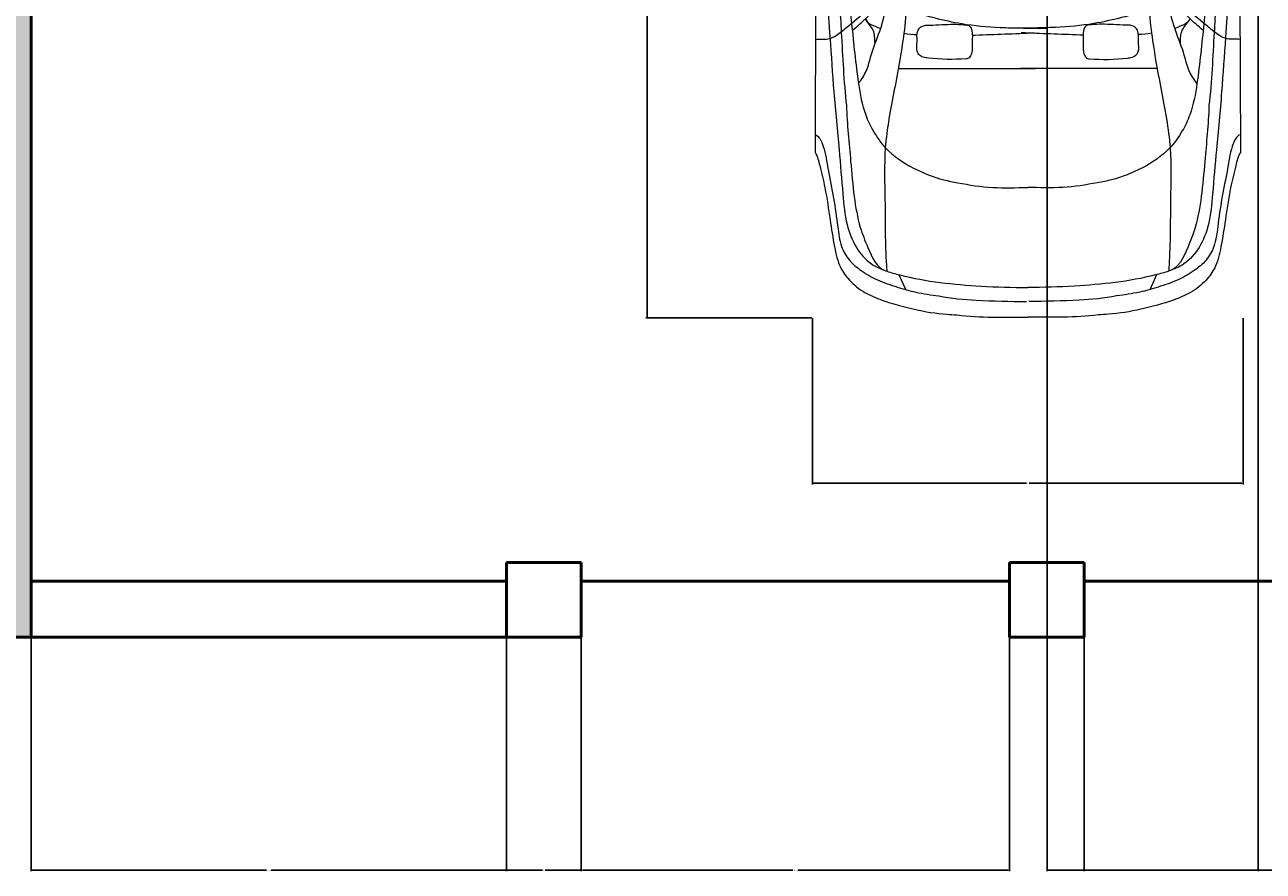
# Model space of a CAD drawing. Units: inches. Extents: x 383 to 970, y 275 to 1088.
# Tile 2 of 11: x 650 to 849, y 275 to 410. Entities that reach past the tile are written whole.
import ezdxf

# ---------------------------------------------------------------- set-up
doc = ezdxf.new("R2010")
doc.units = ezdxf.units.IN
doc.header["$MEASUREMENT"] = 0
for name, color, linetype, lineweight in [('A-ANNO-DIMS', 2, 'Continuous', 18), ('A-COLS', 7, 'Continuous', 50), ('A-EQPM-VEHI', 8, 'Continuous', 13), ('A-WALL', 7, 'Continuous', 50)]:
    doc.layers.add(name, color=color, linetype=linetype, lineweight=lineweight)
doc.layers.add('A-WALL-PATT', color=251, linetype='Continuous', lineweight=13, true_color=0x636466)
doc.styles.get("Standard").update_dxf_attribs({"font": 'arial.ttf'})
doc.dimstyles.get("Standard").update_dxf_attribs({"dimtxt": 0.18, "dimasz": 0.18, "dimexe": 0.18, "dimexo": 0.0625, "dimgap": 0.09, "dimtad": 0, "dimtih": 1, "dimtoh": 1, "dimdec": 4, "dimzin": 0, "dimdsep": 46, "dimtxsty": 'Standard', "dimcen": 0.09, "dimadec": 0, "dimazin": 0, "dimtfac": 1, "dimtdec": 4, "dimtofl": 0, "dimtmove": 0, "dimatfit": 3, "dimfxl": 1, "dimtolj": 1, "dimtzin": 0, "dimarcsym": 0})

# ---------------------------------------------------------------- blocks, each defined once
blk = doc.blocks.new('A$C242571DA')
for p, q in [((1714.3, 1732.5), (3817.1, 1739.9)), ((3474.6, 1401.1), (3474.6, 843)), ((4315.2, 1398), (4377.3, 1370.5)), ((3474.6, 345.6), (3474.6, 903.8)), ((4315.2, 348.7), (4377.3, 376.3)), ((1714.3, 14.2), (3817.1, 6.9))]:
    blk.add_line(p, q)
for points, knots in [([(3356.5, 1739.4), (3354.9, 1719.2), (3360.8, 1678.2), (3324, 1631.5), (3255.4, 1544.3), (3187.1, 1476.2), (3125.2, 1432.2)], [0, 0, 0, 0, 0.0597371, 0.1139981, 0.1672498, 0.3938869, 0.3938869, 0.3938869, 0.3938869]), ([(3745.3, 1736.8), (3748.5, 1730.1), (3764.2, 1717.1), (3811.5, 1698.6), (3894.7, 1686.7), (4002.9, 1663.2), (4107.9, 1648.7), (4195.8, 1638.3), (4258.6, 1603.2), (4302.1, 1549.7), (4339.9, 1483.8), (4365.2, 1407.6), (4389.6, 1324.4), (4397.9, 1266.9), (4401.8, 1235.2)], [0, 0, 0, 0, 0.0219205, 0.0572122, 0.1522539, 0.2718866, 0.3894011, 0.4710097, 0.5346344, 0.5986698, 0.6733118, 0.758696, 0.8351341, 0.9293726, 0.9293726, 0.9293726, 0.9293726]), ([(3817.1, 1739.9), (3833.2, 1729.7), (3882.9, 1718.2), (3973.3, 1695.2), (4085.1, 1680.5), (4193.8, 1662.8), (4280.6, 1644.3), (4343.9, 1598.1), (4390, 1540.3), (4427.4, 1448.7), (4457.8, 1336.6), (4475.7, 1233.4), (4478.4, 1175.1), (4479.3, 1161.6)], [0, 0, 0, 0, 0.056668, 0.14946, 0.28161, 0.392935, 0.481686, 0.542967, 0.622845, 0.69797, 0.833643, 0.965665, 1.00577, 1.00577, 1.00577, 1.00577]), ([(2984.7, 1695.8), (3051, 1695.6), (3172.1, 1691.3), (3367.4, 1677.6), (3575.2, 1664.3), (3788.2, 1643.6), (3968, 1628.1), (4103.8, 1616.8), (4203.6, 1578.1), (4271.8, 1519.5), (4300.6, 1452.1), (4341.7, 1305.3), (4361.8, 1111.2), (4367.5, 936.8), (4367.5, 873.4)], [0, 0, 0, 0, 0.198873, 0.363323, 0.587433, 0.823543, 1.004622, 1.129816, 1.230113, 1.320655, 1.388577, 1.443334, 1.771447, 1.958652, 1.958652, 1.958652, 1.958652]), ([(2695.2, 1655.3), (2829.9, 1655.3), (3041.2, 1651.4), (3351.3, 1630.7), (3527.5, 1623.2), (3626.6, 1612)], [0, 0, 0, 0, 0.4042759, 0.6333827, 0.9326252, 0.9326252, 0.9326252, 0.9326252]), ([(3535.9, 1563.1), (3520.1, 1550.9), (3484.4, 1526.1), (3408.2, 1510.9), (3323.4, 1473.1), (3207.9, 1445), (3072.6, 1422.2), (2866.9, 1404.6), (2626.4, 1412.9), (2396.7, 1410.8), (2200.9, 1416.9), (2001.3, 1438.2), (1732.1, 1525.9), (1527.9, 1578.9), (1407.5, 1610.7)], [0, 0, 0, 0, 0.05975, 0.126928, 0.230034, 0.336675, 0.482225, 0.641324, 0.954906, 1.203173, 1.330375, 1.542773, 1.802261, 2.175545, 2.175545, 2.175545, 2.175545]), ([(2861.6, 1607.5), (2921.1, 1607.3), (3047.2, 1600.8), (3191.4, 1602), (3356.6, 1584.1), (3498.3, 1570.6), (3623.2, 1549.4), (3664.1, 1533.3)], [0, 0, 0, 0, 0.1783018, 0.3787173, 0.431954, 0.6762374, 0.8077184, 0.8077184, 0.8077184, 0.8077184]), ([(3319, 1587.1), (3303.3, 1568.1), (3256.9, 1516.7), (3206.7, 1467.3), (3171.4, 1439.5)], [0, 0, 0, 0, 1.868162, 5.271297, 5.271297, 5.271297, 5.271297]), ([(3626.6, 1612), (3702.5, 1609.1), (3826.2, 1596.8), (3991.4, 1583.2), (4111.7, 1562.4), (4212.2, 1522.7), (4290.4, 1488), (4300.7, 1447.5)], [0, 0, 0, 0, 0.2277977, 0.3719478, 0.4996814, 0.5863441, 0.709615, 0.709615, 0.709615, 0.709615]), ([(3275.5, 1532.8), (3287.5, 1528.3), (3299.8, 1504.9), (3308.4, 1482.5), (3311.7, 1472.6)], [0, 0, 0, 0, 0.983949, 1.771691, 1.771691, 1.771691, 1.771691]), ([(3372.2, 1495.3), (3354.4, 1496.8), (3316, 1494.7), (3291.6, 1525.8), (3275.5, 1532.8)], [0, 0, 0, 0, 0.0535488, 0.1060573, 0.1060573, 0.1060573, 0.1060573]), ([(3664.1, 1533.3), (3687, 1526), (3734.8, 1502.3), (3816.7, 1444.8), (3884.1, 1342.9), (3925.1, 1239.9), (3937.3, 1177), (3940.4, 1157.6)], [0, 0, 0, 0, 0.0720749, 0.1581284, 0.2958089, 0.4262456, 0.4842292, 0.4842292, 0.4842292, 0.4842292]), ([(1909.8, 1424.9), (1933.5, 1418.7), (1995.6, 1407.6), (2094.4, 1385.8), (2211.8, 1377.1), (2419, 1366.9), (2704.7, 1366.5), (3032.7, 1354.2), (3316.2, 1371), (3558.7, 1415.9), (3789.1, 1461.7), (4028.9, 1452.9), (4196.2, 1455.2), (4292.7, 1447.9), (4300.7, 1447.5)], [0, 0, 0, 0, 0.073325, 0.188896, 0.303039, 0.425821, 0.811242, 1.159737, 1.41058, 1.660623, 1.899627, 2.11145, 2.377727, 2.401703, 2.401703, 2.401703, 2.401703]), ([(3231.5, 1368.3), (3240.8, 1356.2), (3253.1, 1315.7), (3271.9, 1240.7), (3297.9, 1127.9), (3310.5, 974.6), (3311.2, 858.3), (3311.6, 794.4)], [0, 0, 0, 0, 0.0451009, 0.1211996, 0.2308505, 0.385263, 0.5739042, 0.5739042, 0.5739042, 0.5739042]), ([(3294.8, 1174.5), (3294.8, 1207.4), (3299.6, 1249.5), (3298.3, 1303.9), (3326.3, 1329), (3363.9, 1320.7), (3399.3, 1329.3), (3422.1, 1315.7), (3430.7, 1297.9), (3438.7, 1234.2), (3439.6, 1174.4), (3434.7, 1112.2), (3418.9, 1102), (3395.9, 1098.6), (3362.6, 1100.9), (3331.1, 1096.6), (3298.8, 1107.6), (3297.3, 1140.3), (3294.8, 1160.9), (3294.8, 1174.5)], [0, 0, 0, 0, 0.0969044, 0.1295913, 0.1506192, 0.1985921, 0.2360698, 0.2557908, 0.2719711, 0.2929882, 0.44406, 0.4519132, 0.4720918, 0.4918599, 0.5228758, 0.5707096, 0.5892096, 0.6145759, 0.654681, 0.654681, 0.654681, 0.654681]), ([(4401.8, 1235.2), (4411.9, 1185.3), (4421.6, 1065.8), (4424.1, 946.5), (4424.1, 878)], [0, 0, 0, 0, 0.1502861, 0.3522699, 0.3522699, 0.3522699, 0.3522699]), ([(3940.4, 1157.6), (3949.9, 1111), (3964.3, 1016.4), (3960.5, 921), (3959.8, 873.4)], [0, 0, 0, 0, 0.140379, 0.2808468, 0.2808468, 0.2808468, 0.2808468]), ([(3339.2, 1099), (3339.1, 1094.8), (3336.4, 1010.6), (3333.2, 926.3), (3330, 846.2)], [11.235438, 11.235438, 11.235438, 11.235438, 11.552536, 17.586883, 17.586883, 17.586883, 17.586883]), ([(3231.5, 378.5), (3240.8, 390.5), (3253.1, 431), (3271.9, 506.1), (3297.9, 618.9), (3310.5, 772.1), (3311.2, 888.4), (3311.6, 952.4)], [0, 0, 0, 0, 0.0451009, 0.1211996, 0.2308505, 0.385263, 0.5739042, 0.5739042, 0.5739042, 0.5739042]), ([(2984.7, 51), (3051, 51.1), (3172.1, 55.5), (3367.4, 69.2), (3575.2, 82.5), (3788.2, 103.1), (3968, 118.7), (4103.8, 130), (4203.6, 168.6), (4271.8, 227.3), (4300.6, 294.7), (4341.7, 441.5), (4361.8, 635.5), (4367.5, 809.9), (4367.5, 873.4)], [0, 0, 0, 0, 0.198873, 0.363323, 0.587433, 0.823543, 1.004622, 1.129816, 1.230113, 1.320655, 1.388577, 1.443334, 1.771447, 1.958652, 1.958652, 1.958652, 1.958652]), ([(3339.2, 647.8), (3339.1, 652), (3336.4, 736.2), (3333.2, 820.5), (3330, 900.6)], [11.235438, 11.235438, 11.235438, 11.235438, 11.552536, 17.586883, 17.586883, 17.586883, 17.586883]), ([(3940.4, 589.1), (3949.9, 635.7), (3964.3, 730.4), (3960.5, 825.8), (3959.8, 873.4)], [0, 0, 0, 0, 0.140379, 0.2808468, 0.2808468, 0.2808468, 0.2808468]), ([(4401.8, 511.5), (4411.9, 561.5), (4421.6, 681), (4424.1, 800.3), (4424.1, 868.8)], [0, 0, 0, 0, 0.1502861, 0.3522699, 0.3522699, 0.3522699, 0.3522699]), ([(3294.8, 572.3), (3294.8, 539.4), (3299.6, 497.2), (3298.3, 442.9), (3326.3, 417.8), (3363.9, 426), (3399.3, 417.5), (3422.1, 431), (3430.7, 448.9), (3438.7, 512.5), (3439.6, 572.4), (3434.7, 634.6), (3418.9, 644.7), (3395.9, 648.2), (3362.6, 645.9), (3331.1, 650.1), (3298.8, 639.2), (3297.3, 606.5), (3294.8, 585.9), (3294.8, 572.3)], [0, 0, 0, 0, 0.0969044, 0.1295913, 0.1506192, 0.1985921, 0.2360698, 0.2557908, 0.2719711, 0.2929882, 0.44406, 0.4519132, 0.4720918, 0.4918599, 0.5228758, 0.5707096, 0.5892096, 0.6145759, 0.654681, 0.654681, 0.654681, 0.654681]), ([(3664.1, 213.5), (3687, 220.8), (3734.8, 244.4), (3816.7, 302), (3884.1, 403.8), (3925.1, 506.9), (3937.3, 569.7), (3940.4, 589.1)], [0, 0, 0, 0, 0.0720749, 0.1581284, 0.2958089, 0.4262456, 0.4842292, 0.4842292, 0.4842292, 0.4842292]), ([(3817.1, 6.9), (3833.2, 17), (3882.9, 28.6), (3973.3, 51.5), (4085.1, 66.3), (4193.8, 84), (4280.6, 102.4), (4343.9, 148.6), (4390, 206.4), (4427.4, 298), (4457.8, 410.1), (4475.7, 513.3), (4478.4, 571.6), (4479.3, 585.2)], [0, 0, 0, 0, 0.056668, 0.14946, 0.28161, 0.392935, 0.481686, 0.542967, 0.622845, 0.69797, 0.833643, 0.965665, 1.00577, 1.00577, 1.00577, 1.00577]), ([(3745.3, 10), (3748.5, 16.7), (3764.2, 29.7), (3811.5, 48.1), (3894.7, 60.1), (4002.9, 83.6), (4107.9, 98), (4195.8, 108.4), (4258.6, 143.5), (4302.1, 197), (4339.9, 262.9), (4365.2, 339.2), (4389.6, 422.4), (4397.9, 479.8), (4401.8, 511.5)], [0, 0, 0, 0, 0.0219205, 0.0572122, 0.1522539, 0.2718866, 0.3894011, 0.4710097, 0.5346344, 0.5986698, 0.6733118, 0.758696, 0.8351341, 0.9293726, 0.9293726, 0.9293726, 0.9293726]), ([(1909.8, 321.9), (1933.5, 328.1), (1995.6, 339.2), (2094.4, 361), (2211.8, 369.6), (2419, 379.8), (2704.7, 380.3), (3032.7, 392.6), (3316.2, 375.8), (3558.7, 330.9), (3789.1, 285.1), (4028.9, 293.9), (4196.2, 291.5), (4292.7, 298.8), (4300.7, 299.2)], [0, 0, 0, 0, 0.073325, 0.188896, 0.303039, 0.425821, 0.811242, 1.159737, 1.41058, 1.660623, 1.899627, 2.11145, 2.377727, 2.401703, 2.401703, 2.401703, 2.401703]), ([(3535.9, 183.7), (3520.1, 195.9), (3484.4, 220.6), (3408.2, 235.8), (3323.4, 273.7), (3207.9, 301.8), (3072.6, 324.6), (2866.9, 342.1), (2626.4, 333.8), (2396.7, 335.9), (2200.9, 329.9), (2001.3, 308.6), (1732.1, 220.8), (1527.9, 167.8), (1407.5, 136)], [0, 0, 0, 0, 0.05975, 0.126928, 0.230034, 0.336675, 0.482225, 0.641324, 0.954906, 1.203173, 1.330375, 1.542773, 1.802261, 2.175545, 2.175545, 2.175545, 2.175545]), ([(3356.5, 7.4), (3354.9, 27.5), (3360.8, 68.5), (3324, 115.2), (3255.4, 202.5), (3187.1, 270.5), (3125.2, 314.6)], [0, 0, 0, 0, 0.0597371, 0.1139981, 0.1672498, 0.3938869, 0.3938869, 0.3938869, 0.3938869]), ([(3319, 159.7), (3303.3, 178.6), (3256.9, 230), (3206.7, 279.5), (3171.4, 307.2)], [0, 0, 0, 0, 1.868162, 5.271297, 5.271297, 5.271297, 5.271297]), ([(3275.5, 214), (3287.5, 218.5), (3299.8, 241.9), (3308.4, 264.3), (3311.7, 274.2)], [0, 0, 0, 0, 0.983949, 1.771691, 1.771691, 1.771691, 1.771691]), ([(3626.6, 134.7), (3702.5, 137.7), (3826.2, 149.9), (3991.4, 163.5), (4111.7, 184.4), (4212.2, 224.1), (4290.4, 258.8), (4300.7, 299.2)], [0, 0, 0, 0, 0.2277977, 0.3719478, 0.4996814, 0.5863441, 0.709615, 0.709615, 0.709615, 0.709615]), ([(2861.6, 139.2), (2921.1, 139.4), (3047.2, 146), (3191.4, 144.8), (3356.6, 162.6), (3498.3, 176.1), (3623.2, 197.4), (3664.1, 213.5)], [0, 0, 0, 0, 0.1783018, 0.3787173, 0.431954, 0.6762374, 0.8077184, 0.8077184, 0.8077184, 0.8077184]), ([(3372.2, 251.5), (3354.4, 249.9), (3316, 252), (3291.6, 220.9), (3275.5, 214)], [0, 0, 0, 0, 0.0535488, 0.1060573, 0.1060573, 0.1060573, 0.1060573]), ([(2695.2, 91.4), (2829.9, 91.5), (3041.2, 95.4), (3351.3, 116.1), (3527.5, 123.5), (3626.6, 134.7)], [0, 0, 0, 0, 0.4042759, 0.6333827, 0.9326252, 0.9326252, 0.9326252, 0.9326252])]:
    blk.add_open_spline(points, degree=3, knots=knots)
for points in [[(3331.9, 1378.1), (3334.2, 1360.4), (3335.9, 1342.5), (3337.3, 1324.5)], [(4479.3, 1161.6), (4491, 1066.2), (4488, 969.5), (4488, 873.4)], [(4479.3, 585.2), (4491, 680.6), (4488, 777.3), (4488, 873.4)], [(3331.9, 368.6), (3334.2, 386.4), (3335.9, 404.3), (3337.3, 422.2)]]:
    blk.add_open_spline(points, degree=3)
blk = doc.blocks.new('*D31')
at = {"layer": 'A-ANNO-DIMS', "color": 0, "lineweight": -2, "transparency": 16777216}
for p, q in [((776.51, 540.18), (749.87, 540.18)), ((750.05, 540), (750.05, 451.95)), ((750.05, 363.55), (750.05, 451.59)), ((776.51, 363.37), (749.87, 363.37))]:
    blk.add_line(p, q, dxfattribs=at)
at = {"layer": 'A-ANNO-DIMS', "color": 0, "transparency": 16777216}
for points in [[(750.02, 540), (750.08, 540), (750.05, 540.18)], [(750.02, 363.55), (750.08, 363.55), (750.05, 363.37)]]:
    blk.add_solid(points, dxfattribs=at)
at = {"layer": 'Defpoints', "color": 0, "transparency": 16777216}
for p in [(776.57, 540.18), (750.05, 363.37), (776.57, 363.37)]:
    blk.add_point(p, dxfattribs=at)
at = {"layer": 'A-ANNO-DIMS', "color": 0, "transparency": 16777216, "insert": (750.05, 451.77), "char_height": 0.18, "attachment_point": 5}
blk.add_mtext('\\A1;CAR 177', dxfattribs=at)
blk = doc.blocks.new('*D32')
at = {"layer": 'A-ANNO-DIMS', "color": 0, "lineweight": -2, "transparency": 16777216}
for p, q in [((776.57, 363.3), (776.57, 336.66)), ((845.67, 363.3), (845.67, 336.66)), ((776.75, 336.84), (810.9, 336.84)), ((845.49, 336.84), (811.34, 336.84))]:
    blk.add_line(p, q, dxfattribs=at)
at = {"layer": 'A-ANNO-DIMS', "color": 0, "transparency": 16777216}
for points in [[(776.75, 336.87), (776.75, 336.81), (776.57, 336.84)], [(845.49, 336.87), (845.49, 336.81), (845.67, 336.84)]]:
    blk.add_solid(points, dxfattribs=at)
at = {"layer": 'Defpoints', "color": 0, "transparency": 16777216}
for p in [(776.57, 363.37), (845.67, 363.37), (845.67, 336.84)]:
    blk.add_point(p, dxfattribs=at)
at = {"layer": 'A-ANNO-DIMS', "color": 0, "transparency": 16777216, "insert": (811.12, 336.84), "char_height": 0.18, "attachment_point": 5}
blk.add_mtext('\\A1;69', dxfattribs=at)
blk = doc.blocks.new('*D42')
at = {"layer": 'A-ANNO-DIMS', "color": 0, "lineweight": -2, "transparency": 16777216}
for p, q in [((651.24, 312.07), (651.24, 274.61)), ((727.5, 312.07), (727.5, 274.61)), ((651.42, 274.79), (688.98, 274.79)), ((727.32, 274.79), (689.76, 274.79))]:
    blk.add_line(p, q, dxfattribs=at)
at = {"layer": 'A-ANNO-DIMS', "color": 0, "transparency": 16777216}
for points in [[(651.42, 274.82), (651.42, 274.76), (651.24, 274.79)], [(727.32, 274.82), (727.32, 274.76), (727.5, 274.79)]]:
    blk.add_solid(points, dxfattribs=at)
at = {"layer": 'Defpoints', "color": 0, "transparency": 16777216}
for p in [(651.24, 312.14), (727.5, 312.14), (727.5, 274.79)]:
    blk.add_point(p, dxfattribs=at)
at = {"layer": 'A-ANNO-DIMS', "color": 0, "transparency": 16777216, "insert": (689.37, 274.79), "char_height": 0.18, "attachment_point": 5}
blk.add_mtext('\\A1;76.26', dxfattribs=at)
blk = doc.blocks.new('*D43')
at = {"layer": 'A-ANNO-DIMS', "color": 0, "lineweight": -2, "transparency": 16777216}
for p, q in [((727.5, 312.07), (727.5, 274.61)), ((739.5, 312.07), (739.5, 274.61)), ((727.68, 274.79), (733.29, 274.79)), ((739.32, 274.79), (733.71, 274.79))]:
    blk.add_line(p, q, dxfattribs=at)
at = {"layer": 'A-ANNO-DIMS', "color": 0, "transparency": 16777216}
for points in [[(727.68, 274.82), (727.68, 274.76), (727.5, 274.79)], [(739.32, 274.82), (739.32, 274.76), (739.5, 274.79)]]:
    blk.add_solid(points, dxfattribs=at)
at = {"layer": 'Defpoints', "color": 0, "transparency": 16777216}
for p in [(727.5, 312.14), (739.5, 312.14), (739.5, 274.79)]:
    blk.add_point(p, dxfattribs=at)
at = {"layer": 'A-ANNO-DIMS', "color": 0, "transparency": 16777216, "insert": (733.5, 274.79), "char_height": 0.18, "attachment_point": 5}
blk.add_mtext('\\A1;12', dxfattribs=at)
blk = doc.blocks.new('*D44')
at = {"layer": 'A-ANNO-DIMS', "color": 0, "lineweight": -2, "transparency": 16777216}
for p, q in [((739.5, 312.07), (739.5, 274.61)), ((808.18, 312.07), (808.18, 274.61)), ((739.68, 274.79), (773.45, 274.79)), ((808, 274.79), (774.24, 274.79))]:
    blk.add_line(p, q, dxfattribs=at)
at = {"layer": 'A-ANNO-DIMS', "color": 0, "transparency": 16777216}
for points in [[(739.68, 274.82), (739.68, 274.76), (739.5, 274.79)], [(808, 274.82), (808, 274.76), (808.18, 274.79)]]:
    blk.add_solid(points, dxfattribs=at)
at = {"layer": 'Defpoints', "color": 0, "transparency": 16777216}
for p in [(739.5, 312.14), (808.18, 312.14), (808.18, 274.79)]:
    blk.add_point(p, dxfattribs=at)
at = {"layer": 'A-ANNO-DIMS', "color": 0, "transparency": 16777216, "insert": (773.84, 274.79), "char_height": 0.18, "attachment_point": 5}
blk.add_mtext('\\A1;68.68', dxfattribs=at)
blk = doc.blocks.new('*D45')
at = {"layer": 'A-ANNO-DIMS', "color": 0, "lineweight": -2, "transparency": 16777216}
for p, q in [((820.18, 312.07), (820.18, 274.61)), ((923.24, 312.07), (923.24, 274.61)), ((820.36, 274.79), (871.26, 274.79)), ((923.06, 274.79), (872.17, 274.79))]:
    blk.add_line(p, q, dxfattribs=at)
at = {"layer": 'A-ANNO-DIMS', "color": 0, "transparency": 16777216}
for points in [[(820.36, 274.82), (820.36, 274.76), (820.18, 274.79)], [(923.06, 274.82), (923.06, 274.76), (923.24, 274.79)]]:
    blk.add_solid(points, dxfattribs=at)
at = {"layer": 'Defpoints', "color": 0, "transparency": 16777216}
for p in [(820.18, 312.14), (923.24, 312.14), (923.24, 274.79)]:
    blk.add_point(p, dxfattribs=at)
at = {"layer": 'A-ANNO-DIMS', "color": 0, "transparency": 16777216, "insert": (871.71, 274.79), "char_height": 0.18, "attachment_point": 5}
blk.add_mtext('\\A1;103.06', dxfattribs=at)
blk = doc.blocks.new('*D57')
at = {"layer": 'A-ANNO-DIMS', "color": 0, "lineweight": -2, "transparency": 16777216}
for p, q in [((814.24, 615.07), (814.24, 274.61)), ((848.09, 615.07), (848.09, 274.61)), ((814.42, 274.79), (830.77, 274.79)), ((847.91, 274.79), (831.56, 274.79))]:
    blk.add_line(p, q, dxfattribs=at)
at = {"layer": 'A-ANNO-DIMS', "color": 0, "transparency": 16777216}
for points in [[(814.42, 274.82), (814.42, 274.76), (814.24, 274.79)], [(847.91, 274.82), (847.91, 274.76), (848.09, 274.79)]]:
    blk.add_solid(points, dxfattribs=at)
at = {"layer": 'Defpoints', "color": 0, "transparency": 16777216}
for p in [(814.24, 615.14), (848.09, 615.14), (848.09, 274.79)]:
    blk.add_point(p, dxfattribs=at)
at = {"layer": 'A-ANNO-DIMS', "color": 0, "transparency": 16777216, "insert": (831.16, 274.79), "char_height": 0.18, "attachment_point": 5}
blk.add_mtext('\\A1;33.85', dxfattribs=at)

msp = doc.modelspace()

# ---------------------------------------------------------------- hatches: boundary and pattern name
at = {"layer": 'A-WALL-PATT'}
h = msp.add_hatch(color=256, dxfattribs=at)
h.dxf.hatch_style = 1
h.paths.add_polyline_path([(651.24, 321.1365), (651.24, 417.1365), (735.24, 417.1365), (735.24, 491.9233), (726.24, 491.9233), (726.24, 426.1365), (582.24, 426.1365), (582.24, 606.1365), (687.24, 606.1365), (687.24, 615.1365), (573.24, 615.1365), (573.24, 546.1365), (570.24, 546.1365), (570.24, 537.1365), (573.24, 537.1365), (573.24, 414.1365), (582.24, 414.1365), (582.24, 417.1365), (642.24, 417.1365), (642.24, 321.1365), (621.6203, 321.1365), (621.6203, 312.1365), (651.24, 312.1365)], flags=17)
h.paths.add_polyline_path([(597.6203, 321.1365), (582.24, 321.1365), (582.24, 390.1365), (573.24, 390.1365), (573.24, 321.1365), (570.24, 321.1365), (570.24, 312.1365), (573.24, 312.1365), (597.6203, 312.1365)], flags=16)
h.paths.add_polyline_path([(534.24, 321.1365), (500.8868, 321.1365), (500.8868, 312.1365), (534.24, 312.1365)], flags=17)
h.paths.add_polyline_path([(735.24, 606.1365), (738.24, 606.1365), (738.24, 615.1365), (723.24, 615.1365), (723.24, 606.1365), (726.24, 606.1365), (726.24, 551.9233), (735.24, 551.9233)], flags=17)
h.paths.add_polyline_path([(848.0899, 615.1365), (814.24, 615.1365), (814.24, 689.38), (805.24, 689.38), (805.24, 615.1365), (802.24, 615.1365), (802.24, 606.1365), (848.0899, 606.1365)], flags=17)
h.paths.add_polyline_path([(530.24, 615.1365), (498.24, 615.1365), (498.24, 646.5351), (489.24, 646.5351), (489.24, 615.1365), (466.771, 615.1365), (466.771, 606.1365), (521.24, 606.1365), (521.24, 603.1365), (530.24, 603.1365), (530.24, 606.1365)], flags=17)
h.paths.add_polyline_path([(498.24, 744.1365), (489.24, 744.1365), (489.24, 706.5351), (498.24, 706.5351)], flags=17)
h.paths.add_polyline_path([(715.24, 792.1365), (598.24, 792.1365), (598.24, 972.1365), (636.5058, 972.1365), (636.5058, 981.1365), (589.24, 981.1365), (589.24, 972.1365), (589.24, 792.1365), (586.24, 792.1365), (586.24, 783.1365), (589.24, 783.1365), (715.24, 783.1365)], flags=17)
h.paths.add_polyline_path([(763.24, 981.1365), (696.5058, 981.1365), (696.5058, 972.1365), (754.24, 972.1365), (754.24, 792.1365), (751.24, 792.1365), (751.24, 783.1365), (754.24, 783.1365), (764.24, 783.1365), (764.24, 792.1365), (763.24, 792.1365)], flags=17)
h.paths.add_polyline_path([(815.24, 1001.9492), (806.24, 1001.9492), (806.24, 972.1365), (818.24, 972.1365), (818.24, 981.1365), (815.24, 981.1365)], flags=17)
h.paths.add_polyline_path([(546.24, 1004.0336), (537.24, 1004.0336), (537.24, 981.1365), (534.24, 981.1365), (534.24, 972.1365), (537.24, 972.1365), (546.24, 972.1365), (546.24, 981.1365)], flags=17)
h.paths.add_polyline_path([(884.0899, 606.1365), (932.24, 606.1365), (932.24, 1050.1365), (420.24, 1050.1365), (420.24, 312.1365), (440.8868, 312.1365), (440.8868, 321.1365), (429.24, 321.1365), (429.24, 537.1365), (538.24, 537.1365), (538.24, 546.1365), (530.24, 546.1365), (530.24, 579.1365), (521.24, 579.1365), (521.24, 546.1365), (429.24, 546.1365), (429.24, 606.1365), (442.771, 606.1365), (442.771, 615.1365), (429.24, 615.1365), (429.24, 783.1365), (489.24, 783.1365), (489.24, 780.1365), (498.24, 780.1365), (498.24, 783.1365), (550.24, 783.1365), (550.24, 792.1365), (429.24, 792.1365), (429.24, 972.1365), (510.24, 972.1365), (510.24, 981.1365), (429.24, 981.1365), (429.24, 1041.1365), (537.24, 1041.1365), (537.24, 1028.0336), (546.24, 1028.0336), (546.24, 1041.1365), (806.24, 1041.1365), (806.24, 1025.9492), (815.24, 1025.9492), (815.24, 1041.1365), (923.24, 1041.1365), (923.24, 981.1365), (842.24, 981.1365), (842.24, 972.1365), (923.24, 972.1365), (923.24, 792.1365), (800.24, 792.1365), (800.24, 783.1365), (805.24, 783.1365), (805.24, 725.38), (814.24, 725.38), (814.24, 783.1365), (923.24, 783.1365), (923.24, 615.1365), (884.0899, 615.1365)])

# ---------------------------------------------------------------- linework, layer by layer
at = {"layer": 'A-COLS'}
for p, q in [((727.5016, 312.1365), (727.5016, 324.1365)), ((727.5016, 324.1365), (739.5016, 324.1365)), ((739.5016, 324.1365), (739.5016, 312.1365)), ((808.1849, 312.1365), (808.1849, 324.1365)), ((808.1849, 324.1365), (820.1849, 324.1365)), ((820.1849, 324.1365), (820.1849, 312.1365)), ((808.1849, 312.1365), (820.1849, 312.1365))]:
    msp.add_line(p, q, dxfattribs=at)
at = {"layer": 'A-WALL'}
for p, q in [((651.24, 417.1365), (651.24, 321.1365)), ((651.24, 321.1365), (727.5016, 321.1365)), ((651.24, 321.1365), (651.24, 312.1365)), ((739.5016, 321.1365), (808.1849, 321.1365)), ((820.1849, 321.1365), (932.24, 321.1365)), ((569.24, 312.1365), (739.5016, 312.1365))]:
    msp.add_line(p, q, dxfattribs=at)

# ---------------------------------------------------------------- block references
at = {"layer": 'A-EQPM-VEHI', "xscale": 0.0393700787401575, "yscale": 0.0393700787401575, "zscale": 0.0393700787401575, "rotation": 270}
msp.add_blockref('A$C242571DA', (776.7342, 540.1782), dxfattribs=at)

# ---------------------------------------------------------------- dimensions: what is measured, and where the dimension line sits
at = {"layer": 'A-ANNO-DIMS'}
for base, p1, p2, override, picture, middle in [((848.0899, 274.7865), (814.24, 615.1365), (848.0899, 615.1365), {"dimdec": 2, "dimlfac": 1, "dimrnd": 0, "dimzin": 0, "dimdsep": 46, "dimlunit": 2}, '*D57', (831.165, 274.7865)), ((845.666, 336.8433), (776.5724, 363.3653), (845.666, 363.3653), {"dimdec": 0, "dimlfac": 1, "dimrnd": 0, "dimzin": 0, "dimdsep": 46, "dimlunit": 2}, '*D32', (811.1192, 336.8433)), ((727.5016, 274.7865), (651.24, 312.1365), (727.5016, 312.1365), {"dimdec": 2, "dimlfac": 1, "dimrnd": 0, "dimzin": 0, "dimdsep": 46, "dimlunit": 2}, '*D42', (689.3708, 274.7865)), ((739.5016, 274.7865), (727.5016, 312.1365), (739.5016, 312.1365), {"dimdec": 0, "dimlfac": 1, "dimrnd": 0, "dimzin": 0, "dimdsep": 46, "dimlunit": 2}, '*D43', (733.5016, 274.7865)), ((808.1849, 274.7865), (739.5016, 312.1365), (808.1849, 312.1365), {"dimdec": 2, "dimlfac": 1, "dimrnd": 0, "dimzin": 0, "dimdsep": 46, "dimlunit": 2}, '*D44', (773.8433, 274.7865)), ((923.24, 274.7865), (820.1849, 312.1365), (923.24, 312.1365), {"dimdec": 2, "dimlfac": 1, "dimrnd": 0, "dimzin": 0, "dimdsep": 46, "dimlunit": 2}, '*D45', (871.7125, 274.7865))]:
    dim = msp.add_linear_dim(base=base, p1=p1, p2=p2, dimstyle='Standard', override=override, dxfattribs=at)
    dim.commit()
    dim.dimension.update_dxf_attribs({"geometry": picture, "text_midpoint": middle})
dim = msp.add_linear_dim(base=(750.0505, 363.3653), p1=(776.5724, 540.1782), p2=(776.5724, 363.3653), angle=270, text='CAR <>', dimstyle='Standard', override={"dimdec": 0, "dimlfac": 1, "dimrnd": 0, "dimzin": 0, "dimdsep": 46, "dimlunit": 2}, dxfattribs=at)
dim.commit()
dim.dimension.update_dxf_attribs({"geometry": '*D31', "text_midpoint": (750.0505, 451.7717)})

doc.saveas('drawing.dxf')
